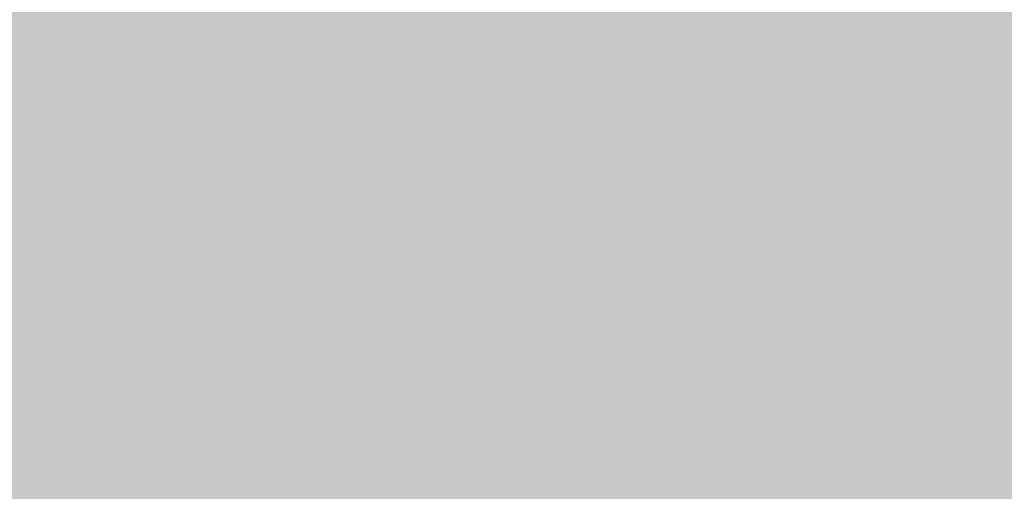
# Model space of a CAD drawing. Units: millimetres. Extents: x 0 to 2267, y 0 to 1823.
# Tile 224 of 256: x 1841.442 to 1842.748, y 1127.775 to 1128.399. Entities that reach past the tile are written whole.
import ezdxf

# ---------------------------------------------------------------- set-up
doc = ezdxf.new("R2010")
doc.units = ezdxf.units.MM
doc.header["$MEASUREMENT"] = 0
doc.layers.add('M-HATC', color=252, linetype='Continuous', lineweight=18)

msp = doc.modelspace()

# ---------------------------------------------------------------- hatches: boundary and pattern name
at = {"layer": 'M-HATC'}
h = msp.add_hatch(color=256, dxfattribs=at)
h.dxf.hatch_style = 1
h.paths.add_polyline_path([(2055.771, 1603.062), (1381.0868, 1603.062), (1381.0868, 1598.062), (2055.771, 1598.062)])
h.paths.add_polyline_path([(2055.771, 1598.062), (1381.0868, 1598.062), (1381.0868, 1593.062), (2055.771, 1593.062)])
h.paths.add_polyline_path([(2051.3074, 1536.7609), (1385.5504, 1536.7609), (1385.5504, 1526.7609), (1387.5504, 1526.7609), (1388.5366, 1525.0528), (1385.3319, 1521.2335), (1385.3319, 1521.2226), (2050.2542, 1522.7491), (2048.3212, 1525.0528), (2049.3074, 1526.7609), (2051.3074, 1526.7609)])
edge = h.paths.add_edge_path()
edge.add_arc((1847.5345, 1379.1492), 135, 222.603061, 222.890851, ccw=False)
edge.add_line((1748.1663, 1287.7656), (1683.0921, 1287.7656))
edge.add_arc((1583.7239, 1379.1492), 135, 317.109149, 317.396939, ccw=False)
edge.add_arc((1678.9686, 1290.6707), 5, 222.8909, 317.1091, ccw=False)
edge.add_arc((1774.2133, 1379.1492), 135, 222.603061, 222.890851, ccw=False)
edge.add_line((1674.8451, 1287.7656), (1609.7709, 1287.7656))
edge.add_arc((1510.4027, 1379.1492), 135, 317.109149, 317.396939, ccw=False)
edge.add_arc((1605.6474, 1290.6707), 5, 222.8909, 317.1091, ccw=False)
edge.add_arc((1700.8921, 1379.1492), 135, 222.603061, 222.890851, ccw=False)
edge.add_line((1601.5239, 1287.7656), (1536.4497, 1287.7656))
edge.add_arc((1437.0815, 1379.1492), 135, 317.109149, 317.396939, ccw=False)
edge.add_arc((1532.3262, 1290.6707), 5, 222.8909, 317.1091, ccw=False)
edge.add_arc((1627.5709, 1379.1492), 135, 222.603061, 222.890851, ccw=False)
edge.add_line((1528.2027, 1287.7656), (1505.9289, 1287.7656))
edge.add_spline(control_points=[(1505.9289, 1287.7656), (1504.2622, 1287.7656), (1504.2622, 1282.7656), (1505.9289, 1282.7656)], knot_values=[0, 0, 0, 0, 5, 5, 5, 5], degree=3, periodic=0)
edge.add_line((1505.9289, 1282.7656), (1930.9289, 1282.7656))
edge.add_spline(control_points=[(1930.9289, 1282.7656), (1932.5956, 1282.7656), (1932.5956, 1287.7656), (1930.9289, 1287.7656)], knot_values=[0, 0, 0, 0, 5, 5, 5, 5], degree=3, periodic=0)
edge.add_line((1930.9289, 1287.7656), (1903.0557, 1287.7656))
edge.add_arc((1803.6875, 1379.1492), 135, 317.109149, 317.396939, ccw=False)
edge.add_arc((1898.9322, 1290.6707), 5, 222.8909, 317.1091, ccw=False)
edge.add_arc((1994.1769, 1379.1492), 135, 222.603061, 222.890851, ccw=False)
edge.add_line((1894.8087, 1287.7656), (1829.7345, 1287.7656))
edge.add_arc((1730.3663, 1379.1492), 135, 317.109149, 317.396939, ccw=False)
edge.add_arc((1825.611, 1290.6707), 5, 222.8909, 317.1091, ccw=False)
edge.add_arc((1920.8557, 1379.1492), 135, 222.603061, 222.890851, ccw=False)
edge.add_line((1821.4875, 1287.7656), (1756.4133, 1287.7656))
edge.add_arc((1657.0451, 1379.1492), 135, 317.109149, 317.396939, ccw=False)
edge.add_arc((1752.2898, 1290.6707), 5, 222.8909, 317.1091, ccw=False)
edge = h.paths.add_edge_path()
edge.add_spline(control_points=[(1843.4289, 1227.2475), (1845.0956, 1227.2475), (1845.0956, 1232.2475), (1843.4289, 1232.2475)], knot_values=[0, 0, 0, 0, 5, 5, 5, 5], degree=3, periodic=0)
edge.add_line((1843.4289, 1232.2475), (1593.4289, 1232.2475))
edge.add_spline(control_points=[(1593.4289, 1232.2475), (1591.7622, 1232.2475), (1591.7622, 1227.2475), (1593.4289, 1227.2475)], knot_values=[0, 0, 0, 0, 5, 5, 5, 5], degree=3, periodic=0)
edge.add_line((1593.4289, 1227.2475), (1843.4289, 1227.2475))
h.paths.add_polyline_path([(1905.9289, 1127.4171), (1530.9289, 1127.4171, 0.414214), (1520.9289, 1117.4171), (1530.9289, 1117.4171), (1915.9289, 1117.4171, 0.414214)])
edge = h.paths.add_edge_path()
edge.add_arc((1397.0858, 1498.4078), 12.7299, 90.78215, 190.87871, ccw=False)
edge.add_line((1396.912, 1511.1365), (1428.0097, 1511.3488))
edge.add_line((1428.0097, 1511.3488), (1433.0097, 1511.3488))
edge.add_line((1433.0097, 1511.3488), (1434.439, 1511.3488))
edge.add_arc((1419.474, 1498.0804), 20, 41.561, 74.08211)
edge.add_line((1424.9592, 1517.3135), (1399.9351, 1517.2561))
edge.add_spline(control_points=[(1399.9307, 1517.2561), (1399.884, 1517.2131), (1399.8328, 1517.1689), (1399.7774, 1517.1236)], knot_values=[11.567499, 11.567499, 11.567499, 11.567499, 11.814249, 11.814249, 11.814249, 11.814249], degree=3, periodic=0)
edge.add_spline(control_points=[(1399.6328, 1517.0099), (1399.5831, 1516.9721), (1399.5307, 1516.9338), (1399.4759, 1516.8947)], knot_values=[11.167718, 11.167718, 11.167718, 11.167718, 11.365188, 11.365188, 11.365188, 11.365188], degree=3, periodic=0)
edge.add_spline(control_points=[(1399.3398, 1516.8001), (1399.1514, 1516.6719), (1398.9384, 1516.5377), (1398.704, 1516.3994)], knot_values=[10.376405, 10.376405, 10.376405, 10.376405, 11.00994, 11.00994, 11.00994, 11.00994], degree=3, periodic=0)
edge.add_spline(control_points=[(1398.6572, 1516.3719), (1398.5789, 1516.326), (1398.4983, 1516.2797), (1398.4155, 1516.2331)], knot_values=[10.125175, 10.125175, 10.125175, 10.125175, 10.334406, 10.334406, 10.334406, 10.334406], degree=3, periodic=0)
edge.add_spline(control_points=[(1398.2642, 1516.1487), (1398.196, 1516.1111), (1398.1263, 1516.0732), (1398.0555, 1516.0351)], knot_values=[9.832246, 9.832246, 9.832246, 9.832246, 9.999658, 9.999658, 9.999658, 9.999658], degree=3, periodic=0)
edge.add_spline(control_points=[(1397.9987, 1516.0048), (1397.7312, 1515.8621), (1397.446, 1515.7171), (1397.1466, 1515.5714)], knot_values=[9.161808, 9.161808, 9.161808, 9.161808, 9.787769, 9.787769, 9.787769, 9.787769], degree=3, periodic=0)
edge.add_spline(control_points=[(1397.1466, 1515.5714), (1396.8418, 1515.423), (1396.5222, 1515.274), (1396.1914, 1515.1262)], knot_values=[8.524455, 8.524455, 8.524455, 8.524455, 9.161808, 9.161808, 9.161808, 9.161808], degree=3, periodic=0)
edge.add_spline(control_points=[(1396.0777, 1515.0756), (1395.9854, 1515.0348), (1395.8922, 1514.994), (1395.7983, 1514.9534)], knot_values=[8.275193, 8.275193, 8.275193, 8.275193, 8.451726, 8.451726, 8.451726, 8.451726], degree=3, periodic=0)
edge.add_spline(control_points=[(1395.6018, 1514.8691), (1395.4997, 1514.8257), (1395.3968, 1514.7824), (1395.2932, 1514.7394)], knot_values=[7.962917, 7.962917, 7.962917, 7.962917, 8.152764, 8.152764, 8.152764, 8.152764], degree=3, periodic=0)
edge.add_spline(control_points=[(1395.2116, 1514.7057), (1394.8278, 1514.5475), (1394.4345, 1514.3929), (1394.0364, 1514.2442)], knot_values=[7.21254, 7.21254, 7.21254, 7.21254, 7.913148, 7.913148, 7.913148, 7.913148], degree=3, periodic=0)
edge.add_spline(control_points=[(1394.0364, 1514.2442), (1393.7076, 1514.1214), (1393.3754, 1514.0027), (1393.0427, 1513.8895)], knot_values=[6.633733, 6.633733, 6.633733, 6.633733, 7.21254, 7.21254, 7.21254, 7.21254], degree=3, periodic=0)
edge.add_spline(control_points=[(1392.8214, 1513.815), (1392.7198, 1513.7812), (1392.6181, 1513.7479), (1392.5166, 1513.7152)], knot_values=[6.328796, 6.328796, 6.328796, 6.328796, 6.505493, 6.505493, 6.505493, 6.505493], degree=3, periodic=0)
edge.add_spline(control_points=[(1392.5166, 1513.7152), (1392.3187, 1513.6515), (1392.1212, 1513.59), (1391.9244, 1513.531)], knot_values=[5.984605, 5.984605, 5.984605, 5.984605, 6.328796, 6.328796, 6.328796, 6.328796], degree=3, periodic=0)
edge.add_spline(control_points=[(1391.7915, 1513.4915), (1391.3122, 1513.3501), (1390.8384, 1513.2239), (1390.3784, 1513.1171)], knot_values=[5.066697, 5.066697, 5.066697, 5.066697, 5.907055, 5.907055, 5.907055, 5.907055], degree=3, periodic=0)
edge.add_spline(control_points=[(1390.3784, 1513.1171), (1390.1797, 1513.071), (1389.9836, 1513.0284), (1389.7907, 1512.9899)], knot_values=[4.70367, 4.70367, 4.70367, 4.70367, 5.066695, 5.066695, 5.066695, 5.066695], degree=3, periodic=0)
edge.add_spline(control_points=[(1389.422, 1512.9204), (1389.2459, 1512.8892), (1389.0729, 1512.8617), (1388.9036, 1512.8381)], knot_values=[4.130571, 4.130571, 4.130571, 4.130571, 4.469816, 4.469816, 4.469816, 4.469816], degree=3, periodic=0)
edge.add_spline(control_points=[(1388.9036, 1512.8381), (1388.591, 1512.7946), (1388.2911, 1512.7644), (1388.0071, 1512.7494)], knot_values=[3.504031, 3.504031, 3.504031, 3.504031, 4.130571, 4.130571, 4.130571, 4.130571], degree=3, periodic=0)
edge.add_spline(control_points=[(1387.9356, 1512.7459), (1387.8538, 1512.7423), (1387.7733, 1512.74), (1387.6944, 1512.739)], knot_values=[3.268866, 3.268866, 3.268866, 3.268866, 3.451164, 3.451164, 3.451164, 3.451164], degree=3, periodic=0)
edge.add_spline(control_points=[(1387.3351, 1512.7443), (1387.2076, 1512.7499), (1387.0847, 1512.7597), (1386.967, 1512.7739)], knot_values=[2.670686, 2.670686, 2.670686, 2.670686, 2.984, 2.984, 2.984, 2.984], degree=3, periodic=0)
edge.add_spline(control_points=[(1386.8327, 1512.7922), (1386.8209, 1512.7941), (1386.8092, 1512.7959), (1386.7975, 1512.7979)], knot_values=[2.516981, 2.516981, 2.516981, 2.516981, 2.549528, 2.549528, 2.549528, 2.549528], degree=3, periodic=0)
edge.add_spline(control_points=[(1386.4526, 1512.8735), (1386.4257, 1512.881), (1386.3993, 1512.889), (1386.3733, 1512.8972)], knot_values=[2.095869, 2.095869, 2.095869, 2.095869, 2.17941, 2.17941, 2.17941, 2.17941], degree=3, periodic=0)
edge.add_spline(control_points=[(1386.0691, 1513.0189), (1386.0634, 1513.0217), (1386.0577, 1513.0246), (1386.052, 1513.0275)], knot_values=[1.72453, 1.72453, 1.72453, 1.72453, 1.745933, 1.745933, 1.745933, 1.745933], degree=3, periodic=0)
edge.add_arc((1399.474, 1498.0804), 20, 131.82432, 180)
edge.add_arc((1630.3336, 1505.5484), 250.9708, 181.705176, 236.427975)
edge.add_arc((1605.3399, 1483.3044), 218.7822, 238.660829, 243.34961)
edge.add_arc((1647.0911, 1510.3592), 262.8986, 183.129836, 237.853442, ccw=False)
h.paths.add_polyline_path([(1406.5369, 1391.9644, 0.149382), (1491.5506, 1296.4418, -0.129517)], flags=17)
edge = h.paths.add_edge_path()
edge.add_arc((2037.3838, 1498.0804), 20, 0, 48.26587)
edge.add_spline(control_points=[(2050.6973, 1513.0052), (2050.6512, 1512.9847), (2050.6034, 1512.9655), (2050.5539, 1512.9477)], knot_values=[1.835652, 1.835652, 1.835652, 1.835652, 2.000781, 2.000781, 2.000781, 2.000781], degree=3, periodic=0)
edge.add_spline(control_points=[(2050.4616, 1512.9166), (2050.479, 1512.9221), (2050.4963, 1512.9277), (2050.5133, 1512.9335)], knot_values=[2.045477, 2.045477, 2.045477, 2.045477, 2.101389, 2.101389, 2.101389, 2.101389], degree=3, periodic=0)
edge.add_spline(control_points=[(2050.129, 1512.8342), (2050.1984, 1512.8473), (2050.2657, 1512.8623), (2050.3308, 1512.8792)], knot_values=[2.237629, 2.237629, 2.237629, 2.237629, 2.435841, 2.435841, 2.435841, 2.435841], degree=3, periodic=0)
edge.add_spline(control_points=[(2050.0946, 1512.8278), (2050.1061, 1512.8299), (2050.1176, 1512.832), (2050.129, 1512.8342)], knot_values=[2.435841, 2.435841, 2.435841, 2.435841, 2.468321, 2.468321, 2.468321, 2.468321], degree=3, periodic=0)
edge.add_spline(control_points=[(2049.7843, 1512.7851), (2049.8552, 1512.7922), (2049.9243, 1512.8008), (2049.9917, 1512.8109)], knot_values=[2.563852, 2.563852, 2.563852, 2.563852, 2.748541, 2.748541, 2.748541, 2.748541], degree=3, periodic=0)
edge.add_spline(control_points=[(2049.4052, 1512.7617), (2049.5364, 1512.7653), (2049.6629, 1512.773), (2049.7843, 1512.7851)], knot_values=[2.748541, 2.748541, 2.748541, 2.748541, 3.064882, 3.064882, 3.064882, 3.064882], degree=3, periodic=0)
edge.add_spline(control_points=[(2049.1698, 1512.7597), (2049.2336, 1512.7591), (2049.2965, 1512.7594), (2049.3584, 1512.7606)], knot_values=[3.102309, 3.102309, 3.102309, 3.102309, 3.2503, 3.2503, 3.2503, 3.2503], degree=3, periodic=0)
edge.add_spline(control_points=[(2048.8573, 1512.7691), (2048.9638, 1512.7638), (2049.068, 1512.7606), (2049.1698, 1512.7597)], knot_values=[3.2503, 3.2503, 3.2503, 3.2503, 3.486069, 3.486069, 3.486069, 3.486069], degree=3, periodic=0)
edge.add_spline(control_points=[(2048.6924, 1512.7789), (2048.3729, 1512.8009), (2048.0345, 1512.8411), (2047.6817, 1512.897)], knot_values=[3.606429, 3.606429, 3.606429, 3.606429, 4.2989, 4.2989, 4.2989, 4.2989], degree=3, periodic=0)
edge.add_spline(control_points=[(2047.6817, 1512.897), (2047.5458, 1512.9185), (2047.4077, 1512.9424), (2047.2678, 1512.9685)], knot_values=[4.2989, 4.2989, 4.2989, 4.2989, 4.565769, 4.565769, 4.565769, 4.565769], degree=3, periodic=0)
edge.add_spline(control_points=[(2047.2678, 1512.9685), (2047.1449, 1512.9914), (2047.0207, 1513.016), (2046.8951, 1513.0422)], knot_values=[4.565769, 4.565769, 4.565769, 4.565769, 4.799971, 4.799971, 4.799971, 4.799971], degree=3, periodic=0)
edge.add_spline(control_points=[(2046.8951, 1513.0422), (2046.5286, 1513.1188), (2046.1513, 1513.209), (2045.7676, 1513.3107)], knot_values=[4.799971, 4.799971, 4.799971, 4.799971, 5.483718, 5.483718, 5.483718, 5.483718], degree=3, periodic=0)
edge.add_spline(control_points=[(2045.7676, 1513.3107), (2045.3724, 1513.4154), (2044.9704, 1513.5322), (2044.5662, 1513.6588)], knot_values=[5.483718, 5.483718, 5.483718, 5.483718, 6.187866, 6.187866, 6.187866, 6.187866], degree=3, periodic=0)
edge.add_spline(control_points=[(2044.5662, 1513.6588), (2044.4149, 1513.7061), (2044.2633, 1513.7549), (2044.1116, 1513.8048)], knot_values=[6.187866, 6.187866, 6.187866, 6.187866, 6.451551, 6.451551, 6.451551, 6.451551], degree=3, periodic=0)
edge.add_spline(control_points=[(2044.1116, 1513.8048), (2043.9967, 1513.8427), (2043.8817, 1513.8813), (2043.7668, 1513.9205)], knot_values=[6.451551, 6.451551, 6.451551, 6.451551, 6.651434, 6.651434, 6.651434, 6.651434], degree=3, periodic=0)
edge.add_spline(control_points=[(2043.7668, 1513.9205), (2043.3716, 1514.0554), (2042.9774, 1514.1979), (2042.5886, 1514.3458)], knot_values=[6.651434, 6.651434, 6.651434, 6.651434, 7.338879, 7.338879, 7.338879, 7.338879], degree=3, periodic=0)
edge.add_spline(control_points=[(2042.5886, 1514.3458), (2042.1643, 1514.5071), (2041.7465, 1514.6749), (2041.3409, 1514.846)], knot_values=[7.338879, 7.338879, 7.338879, 7.338879, 8.089209, 8.089209, 8.089209, 8.089209], degree=3, periodic=0)
edge.add_spline(control_points=[(2041.3409, 1514.846), (2041.1028, 1514.9465), (2040.869, 1515.0481), (2040.6405, 1515.1502)], knot_values=[8.089209, 8.089209, 8.089209, 8.089209, 8.529587, 8.529587, 8.529587, 8.529587], degree=3, periodic=0)
edge.add_spline(control_points=[(2040.51, 1515.2089), (2040.0824, 1515.4022), (2039.6747, 1515.5971), (2039.295, 1515.7894)], knot_values=[8.613818, 8.613818, 8.613818, 8.613818, 9.44571, 9.44571, 9.44571, 9.44571], degree=3, periodic=0)
edge.add_spline(control_points=[(2039.295, 1515.7894), (2039.0618, 1515.9075), (2038.8391, 1516.0246), (2038.6288, 1516.1398)], knot_values=[9.44571, 9.44571, 9.44571, 9.44571, 9.956404, 9.956404, 9.956404, 9.956404], degree=3, periodic=0)
edge.add_spline(control_points=[(2038.6288, 1516.1398), (2038.5187, 1516.2001), (2038.4121, 1516.2598), (2038.309, 1516.3189)], knot_values=[9.956404, 9.956404, 9.956404, 9.956404, 10.223542, 10.223542, 10.223542, 10.223542], degree=3, periodic=0)
edge.add_spline(control_points=[(2038.309, 1516.3189), (2038.2138, 1516.3735), (2038.1216, 1516.4276), (2038.0328, 1516.481)], knot_values=[10.223542, 10.223542, 10.223542, 10.223542, 10.47051, 10.47051, 10.47051, 10.47051], degree=3, periodic=0)
edge.add_spline(control_points=[(2038.0328, 1516.481), (2037.7855, 1516.6296), (2037.5639, 1516.773), (2037.3722, 1516.909)], knot_values=[10.47051, 10.47051, 10.47051, 10.47051, 11.15767, 11.15767, 11.15767, 11.15767], degree=3, periodic=0)
edge.add_spline(control_points=[(2037.3722, 1516.909), (2037.2789, 1516.9752), (2037.1927, 1517.0396), (2037.1142, 1517.102)], knot_values=[11.15767, 11.15767, 11.15767, 11.15767, 11.49227, 11.49227, 11.49227, 11.49227], degree=3, periodic=0)
edge.add_spline(control_points=[(2036.8564, 1517.3259), (2036.9148, 1517.2692), (2036.9814, 1517.2103), (2037.0557, 1517.1492)], knot_values=[11.577341, 11.577341, 11.577341, 11.577341, 11.91035, 11.91035, 11.91035, 11.91035], degree=3, periodic=0)
edge.add_spline(control_points=[(2036.8074, 1517.3748), (2036.823, 1517.3587), (2036.8393, 1517.3424), (2036.8564, 1517.3259)], knot_values=[11.91035, 11.91035, 11.91035, 11.91035, 12.007402, 12.007402, 12.007402, 12.007402], degree=3, periodic=0)
edge.add_spline(control_points=[(2036.7017, 1517.494), (2036.7104, 1517.483), (2036.7196, 1517.4719), (2036.7291, 1517.4606)], knot_values=[12.184155, 12.184155, 12.184155, 12.184155, 12.255409, 12.255409, 12.255409, 12.255409], degree=3, periodic=0)
edge.add_spline(control_points=[(2036.6159, 1517.6205), (2036.62, 1517.613), (2036.6243, 1517.6055), (2036.6289, 1517.5979)], knot_values=[12.487913, 12.487913, 12.487913, 12.487913, 12.541035, 12.541035, 12.541035, 12.541035], degree=3, periodic=0)
edge.add_spline(control_points=[(2036.5635, 1517.786), (2036.5637, 1517.7794), (2036.5642, 1517.7726), (2036.565, 1517.7658)], knot_values=[12.911761, 12.911761, 12.911761, 12.911761, 12.968286, 12.968286, 12.968286, 12.968286], degree=3, periodic=0)
edge.add_spline(control_points=[(2036.6166, 1517.9304), (2036.6125, 1517.9259), (2036.6086, 1517.9212), (2036.6049, 1517.9165)], knot_values=[13.382527, 13.382527, 13.382527, 13.382527, 13.433791, 13.433791, 13.433791, 13.433791], degree=3, periodic=0)
edge.add_spline(control_points=[(2036.749, 1518.017), (2036.7361, 1518.0116), (2036.7239, 1518.006), (2036.7124, 1518.0002)], knot_values=[13.726299, 13.726299, 13.726299, 13.726299, 13.809928, 13.809928, 13.809928, 13.809928], degree=3, periodic=0)
edge.add_spline(control_points=[(2036.8604, 1518.0528), (2036.8386, 1518.0474), (2036.8181, 1518.0416), (2036.7988, 1518.0353)], knot_values=[13.910887, 13.910887, 13.910887, 13.910887, 14.02153, 14.02153, 14.02153, 14.02153], degree=3, periodic=0)
edge.add_line((2036.9639, 1518.0804), (2032.3838, 1518.0804))
edge.add_line((2032.3838, 1518.0804), (2027.3838, 1518.0804))
edge.add_line((2027.3838, 1518.0804), (2022.3838, 1518.0804))
edge.add_line((2022.3838, 1518.0804), (2017.3838, 1518.0804))
edge.add_arc((2017.3838, 1498.0804), 20, 90, 138.439)
edge.add_line((2002.4188, 1511.3488), (2003.8481, 1511.3488))
edge.add_line((2003.8481, 1511.3488), (2008.8481, 1511.3488))
edge.add_line((2008.8481, 1511.3488), (2039.772, 1511.1377))
edge.add_arc((2039.772, 1498.4078), 12.7299, -10.87871, 90, ccw=False)
edge.add_arc((1789.7668, 1510.3592), 262.8986, 302.146558, 356.870164, ccw=False)
edge.add_arc((1831.5179, 1483.3044), 218.7822, 296.65039, 301.339171)
edge.add_arc((1806.5242, 1505.5484), 250.9708, 303.572025, 358.294824)
h.paths.add_polyline_path([(2030.321, 1391.9644, -0.129517), (1945.3072, 1296.4418, 0.149382)], flags=17)
edge = h.paths.add_edge_path()
edge.add_spline(control_points=[(2037.2464, 1518.0821), (2037.2898, 1518.081), (2037.3355, 1518.0804), (2037.3838, 1518.0804)], knot_values=[0.000012, 0.000012, 0.000012, 0.000012, 0.144754, 0.144754, 0.144754, 0.144754], degree=3, periodic=0)
edge.add_line((2037.3357, 1518.0804), (2037.0096, 1518.0804))
edge.add_spline(control_points=[(2037.0096, 1518.0804), (2036.9822, 1518.0768), (2036.956, 1518.0727), (2036.9312, 1518.0681)], knot_values=[14.13465, 14.13465, 14.13465, 14.13465, 14.247197, 14.247197, 14.247197, 14.247197], degree=3, periodic=0)
edge.add_spline(control_points=[(2036.9312, 1518.0681), (2036.9276, 1518.0674), (2036.9241, 1518.0667), (2036.9205, 1518.0661)], knot_values=[14.118315, 14.118315, 14.118315, 14.118315, 14.13465, 14.13465, 14.13465, 14.13465], degree=3, periodic=0)
edge.add_spline(control_points=[(2036.9205, 1518.0661), (2036.9118, 1518.0644), (2036.9032, 1518.0626), (2036.8948, 1518.0608)], knot_values=[14.078086, 14.078086, 14.078086, 14.078086, 14.118315, 14.118315, 14.118315, 14.118315], degree=3, periodic=0)
edge.add_spline(control_points=[(2036.8948, 1518.0608), (2036.883, 1518.0583), (2036.8716, 1518.0556), (2036.8604, 1518.0528)], knot_values=[14.02153, 14.02153, 14.02153, 14.02153, 14.078086, 14.078086, 14.078086, 14.078086], degree=3, periodic=0)
edge.add_spline(control_points=[(2036.8604, 1518.0528), (2036.8386, 1518.0474), (2036.8181, 1518.0416), (2036.7988, 1518.0353)], knot_values=[13.910887, 13.910887, 13.910887, 13.910887, 14.02153, 14.02153, 14.02153, 14.02153], degree=3, periodic=0)
edge.add_spline(control_points=[(2036.7988, 1518.0353), (2036.7981, 1518.035), (2036.7974, 1518.0348), (2036.7967, 1518.0346)], knot_values=[13.906906, 13.906906, 13.906906, 13.906906, 13.910887, 13.910887, 13.910887, 13.910887], degree=3, periodic=0)
edge.add_spline(control_points=[(2036.7967, 1518.0346), (2036.7882, 1518.0318), (2036.7799, 1518.0289), (2036.7719, 1518.0259)], knot_values=[13.857826, 13.857826, 13.857826, 13.857826, 13.906906, 13.906906, 13.906906, 13.906906], degree=3, periodic=0)
edge.add_spline(control_points=[(2036.7719, 1518.0259), (2036.764, 1518.023), (2036.7564, 1518.02), (2036.749, 1518.017)], knot_values=[13.809928, 13.809928, 13.809928, 13.809928, 13.857826, 13.857826, 13.857826, 13.857826], degree=3, periodic=0)
edge.add_spline(control_points=[(2036.749, 1518.017), (2036.7361, 1518.0116), (2036.7239, 1518.006), (2036.7124, 1518.0002)], knot_values=[13.726299, 13.726299, 13.726299, 13.726299, 13.809928, 13.809928, 13.809928, 13.809928], degree=3, periodic=0)
edge.add_spline(control_points=[(2036.7124, 1518.0002), (2036.7121, 1518), (2036.7118, 1517.9999), (2036.7115, 1517.9997)], knot_values=[13.723993, 13.723993, 13.723993, 13.723993, 13.726299, 13.726299, 13.726299, 13.726299], degree=3, periodic=0)
edge.add_spline(control_points=[(2036.7115, 1517.9997), (2036.7063, 1517.9971), (2036.7013, 1517.9944), (2036.6965, 1517.9917)], knot_values=[13.686536, 13.686536, 13.686536, 13.686536, 13.723993, 13.723993, 13.723993, 13.723993], degree=3, periodic=0)
edge.add_spline(control_points=[(2036.6965, 1517.9917), (2036.6919, 1517.9891), (2036.6874, 1517.9865), (2036.6831, 1517.9839)], knot_values=[13.651251, 13.651251, 13.651251, 13.651251, 13.686536, 13.686536, 13.686536, 13.686536], degree=3, periodic=0)
edge.add_spline(control_points=[(2036.6831, 1517.9839), (2036.6764, 1517.9798), (2036.67, 1517.9757), (2036.6639, 1517.9714)], knot_values=[13.596804, 13.596804, 13.596804, 13.596804, 13.651251, 13.651251, 13.651251, 13.651251], degree=3, periodic=0)
edge.add_spline(control_points=[(2036.6639, 1517.9714), (2036.6636, 1517.9712), (2036.6633, 1517.9709), (2036.6629, 1517.9707)], knot_values=[13.593956, 13.593956, 13.593956, 13.593956, 13.596804, 13.596804, 13.596804, 13.596804], degree=3, periodic=0)
edge.add_spline(control_points=[(2036.6629, 1517.9707), (2036.6603, 1517.9689), (2036.6577, 1517.967), (2036.6552, 1517.9651)], knot_values=[13.570322, 13.570322, 13.570322, 13.570322, 13.593956, 13.593956, 13.593956, 13.593956], degree=3, periodic=0)
edge.add_spline(control_points=[(2036.6552, 1517.9651), (2036.6525, 1517.9631), (2036.6499, 1517.9611), (2036.6474, 1517.9591)], knot_values=[13.545477, 13.545477, 13.545477, 13.545477, 13.570322, 13.570322, 13.570322, 13.570322], degree=3, periodic=0)
edge.add_spline(control_points=[(2036.6474, 1517.9591), (2036.6472, 1517.9589), (2036.6471, 1517.9588), (2036.6469, 1517.9587)], knot_values=[13.543931, 13.543931, 13.543931, 13.543931, 13.545477, 13.545477, 13.545477, 13.545477], degree=3, periodic=0)
edge.add_spline(control_points=[(2036.6469, 1517.9587), (2036.6412, 1517.9541), (2036.6358, 1517.9494), (2036.6307, 1517.9447)], knot_values=[13.488237, 13.488237, 13.488237, 13.488237, 13.543931, 13.543931, 13.543931, 13.543931], degree=3, periodic=0)
edge.add_spline(control_points=[(2036.6307, 1517.9447), (2036.6282, 1517.9423), (2036.6257, 1517.9399), (2036.6233, 1517.9374)], knot_values=[13.460307, 13.460307, 13.460307, 13.460307, 13.488237, 13.488237, 13.488237, 13.488237], degree=3, periodic=0)
edge.add_spline(control_points=[(2036.6233, 1517.9374), (2036.6215, 1517.9356), (2036.6198, 1517.9338), (2036.6181, 1517.932)], knot_values=[13.439712, 13.439712, 13.439712, 13.439712, 13.460307, 13.460307, 13.460307, 13.460307], degree=3, periodic=0)
edge.add_spline(control_points=[(2036.6181, 1517.932), (2036.6176, 1517.9315), (2036.6171, 1517.9309), (2036.6166, 1517.9304)], knot_values=[13.433791, 13.433791, 13.433791, 13.433791, 13.439712, 13.439712, 13.439712, 13.439712], degree=3, periodic=0)
edge.add_spline(control_points=[(2036.6166, 1517.9304), (2036.6125, 1517.9259), (2036.6086, 1517.9212), (2036.6049, 1517.9165)], knot_values=[13.382527, 13.382527, 13.382527, 13.382527, 13.433791, 13.433791, 13.433791, 13.433791], degree=3, periodic=0)
edge.add_spline(control_points=[(2036.6049, 1517.9165), (2036.6026, 1517.9135), (2036.6004, 1517.9104), (2036.5982, 1517.9074)], knot_values=[13.350017, 13.350017, 13.350017, 13.350017, 13.382527, 13.382527, 13.382527, 13.382527], degree=3, periodic=0)
edge.add_spline(control_points=[(2036.5982, 1517.9074), (2036.5972, 1517.9059), (2036.5962, 1517.9043), (2036.5952, 1517.9028)], knot_values=[13.333922, 13.333922, 13.333922, 13.333922, 13.350017, 13.350017, 13.350017, 13.350017], degree=3, periodic=0)
edge.add_spline(control_points=[(2036.5952, 1517.9028), (2036.5945, 1517.9018), (2036.5939, 1517.9009), (2036.5933, 1517.8999)], knot_values=[13.323828, 13.323828, 13.323828, 13.323828, 13.333922, 13.333922, 13.333922, 13.333922], degree=3, periodic=0)
edge.add_spline(control_points=[(2036.5933, 1517.8999), (2036.5905, 1517.8955), (2036.5879, 1517.8909), (2036.5855, 1517.8864)], knot_values=[13.277545, 13.277545, 13.277545, 13.277545, 13.323828, 13.323828, 13.323828, 13.323828], degree=3, periodic=0)
edge.add_spline(control_points=[(2036.5855, 1517.8864), (2036.5836, 1517.8827), (2036.5817, 1517.8789), (2036.5801, 1517.8751)], knot_values=[13.240119, 13.240119, 13.240119, 13.240119, 13.277545, 13.277545, 13.277545, 13.277545], degree=3, periodic=0)
edge.add_spline(control_points=[(2036.5801, 1517.8751), (2036.5795, 1517.8739), (2036.579, 1517.8727), (2036.5785, 1517.8715)], knot_values=[13.228211, 13.228211, 13.228211, 13.228211, 13.240119, 13.240119, 13.240119, 13.240119], degree=3, periodic=0)
edge.add_spline(control_points=[(2036.5785, 1517.8715), (2036.578, 1517.8702), (2036.5774, 1517.869), (2036.5769, 1517.8677)], knot_values=[13.215717, 13.215717, 13.215717, 13.215717, 13.228211, 13.228211, 13.228211, 13.228211], degree=3, periodic=0)
edge.add_spline(control_points=[(2036.5769, 1517.8677), (2036.5755, 1517.864), (2036.5741, 1517.8603), (2036.5729, 1517.8565)], knot_values=[13.179847, 13.179847, 13.179847, 13.179847, 13.215717, 13.215717, 13.215717, 13.215717], degree=3, periodic=0)
edge.add_spline(control_points=[(2036.5729, 1517.8565), (2036.5713, 1517.8515), (2036.5699, 1517.8464), (2036.5687, 1517.8413)], knot_values=[13.132017, 13.132017, 13.132017, 13.132017, 13.179847, 13.179847, 13.179847, 13.179847], degree=3, periodic=0)
edge.add_spline(control_points=[(2036.5687, 1517.8413), (2036.5684, 1517.8402), (2036.5682, 1517.8392), (2036.568, 1517.8382)], knot_values=[13.122482, 13.122482, 13.122482, 13.122482, 13.132017, 13.132017, 13.132017, 13.132017], degree=3, periodic=0)
edge.add_spline(control_points=[(2036.568, 1517.8382), (2036.5676, 1517.8363), (2036.5672, 1517.8345), (2036.5669, 1517.8327)], knot_values=[13.105592, 13.105592, 13.105592, 13.105592, 13.122482, 13.122482, 13.122482, 13.122482], degree=3, periodic=0)
edge.add_spline(control_points=[(2036.5669, 1517.8327), (2036.5662, 1517.8292), (2036.5657, 1517.8257), (2036.5652, 1517.8222)], knot_values=[13.074063, 13.074063, 13.074063, 13.074063, 13.105592, 13.105592, 13.105592, 13.105592], degree=3, periodic=0)
edge.add_spline(control_points=[(2036.5652, 1517.8222), (2036.5652, 1517.8222), (2036.5652, 1517.8222), (2036.5652, 1517.8222)], knot_values=[13.074043, 13.074043, 13.074043, 13.074043, 13.074063, 13.074063, 13.074063, 13.074063], degree=3, periodic=0)
edge.add_spline(control_points=[(2036.5652, 1517.8222), (2036.5644, 1517.8164), (2036.5639, 1517.8106), (2036.5636, 1517.8046)], knot_values=[13.021884, 13.021884, 13.021884, 13.021884, 13.074043, 13.074043, 13.074043, 13.074043], degree=3, periodic=0)
edge.add_spline(control_points=[(2036.5636, 1517.8046), (2036.5636, 1517.804), (2036.5636, 1517.8034), (2036.5635, 1517.8028)], knot_values=[13.01674, 13.01674, 13.01674, 13.01674, 13.021884, 13.021884, 13.021884, 13.021884], degree=3, periodic=0)
edge.add_spline(control_points=[(2036.5635, 1517.8028), (2036.5634, 1517.8005), (2036.5634, 1517.7982), (2036.5634, 1517.7958)], knot_values=[12.996438, 12.996438, 12.996438, 12.996438, 13.01674, 13.01674, 13.01674, 13.01674], degree=3, periodic=0)
edge.add_spline(control_points=[(2036.5634, 1517.7958), (2036.5633, 1517.7926), (2036.5634, 1517.7893), (2036.5635, 1517.786)], knot_values=[12.968286, 12.968286, 12.968286, 12.968286, 12.996438, 12.996438, 12.996438, 12.996438], degree=3, periodic=0)
edge.add_spline(control_points=[(2036.5635, 1517.786), (2036.5637, 1517.7794), (2036.5642, 1517.7726), (2036.565, 1517.7658)], knot_values=[12.911761, 12.911761, 12.911761, 12.911761, 12.968286, 12.968286, 12.968286, 12.968286], degree=3, periodic=0)
edge.add_spline(control_points=[(2036.565, 1517.7658), (2036.565, 1517.7657), (2036.565, 1517.7656), (2036.565, 1517.7656)], knot_values=[12.911017, 12.911017, 12.911017, 12.911017, 12.911761, 12.911761, 12.911761, 12.911761], degree=3, periodic=0)
edge.add_spline(control_points=[(2036.565, 1517.7656), (2036.5654, 1517.7625), (2036.5658, 1517.7593), (2036.5663, 1517.7562)], knot_values=[12.88528, 12.88528, 12.88528, 12.88528, 12.911017, 12.911017, 12.911017, 12.911017], degree=3, periodic=0)
edge.add_spline(control_points=[(2036.5663, 1517.7562), (2036.5667, 1517.7534), (2036.5672, 1517.7506), (2036.5677, 1517.7478)], knot_values=[12.862519, 12.862519, 12.862519, 12.862519, 12.88528, 12.88528, 12.88528, 12.88528], degree=3, periodic=0)
edge.add_spline(control_points=[(2036.5677, 1517.7478), (2036.5678, 1517.7474), (2036.5679, 1517.7469), (2036.568, 1517.7465)], knot_values=[12.858885, 12.858885, 12.858885, 12.858885, 12.862519, 12.862519, 12.862519, 12.862519], degree=3, periodic=0)
edge.add_spline(control_points=[(2036.568, 1517.7465), (2036.5692, 1517.7399), (2036.5707, 1517.7332), (2036.5724, 1517.7264)], knot_values=[12.8053, 12.8053, 12.8053, 12.8053, 12.858885, 12.858885, 12.858885, 12.858885], degree=3, periodic=0)
edge.add_spline(control_points=[(2036.5724, 1517.7264), (2036.5734, 1517.7226), (2036.5745, 1517.7187), (2036.5756, 1517.7149)], knot_values=[12.775176, 12.775176, 12.775176, 12.775176, 12.8053, 12.8053, 12.8053, 12.8053], degree=3, periodic=0)
edge.add_spline(control_points=[(2036.5756, 1517.7149), (2036.5763, 1517.7125), (2036.577, 1517.7102), (2036.5778, 1517.7078)], knot_values=[12.756759, 12.756759, 12.756759, 12.756759, 12.775176, 12.775176, 12.775176, 12.775176], degree=3, periodic=0)
edge.add_spline(control_points=[(2036.5778, 1517.7078), (2036.5781, 1517.7067), (2036.5784, 1517.7057), (2036.5787, 1517.7047)], knot_values=[12.748742, 12.748742, 12.748742, 12.748742, 12.756759, 12.756759, 12.756759, 12.756759], degree=3, periodic=0)
edge.add_spline(control_points=[(2036.5787, 1517.7047), (2036.5808, 1517.6983), (2036.5831, 1517.6919), (2036.5856, 1517.6854)], knot_values=[12.69959, 12.69959, 12.69959, 12.69959, 12.748742, 12.748742, 12.748742, 12.748742], degree=3, periodic=0)
edge.add_spline(control_points=[(2036.5856, 1517.6854), (2036.5876, 1517.68), (2036.5898, 1517.6746), (2036.5921, 1517.6692)], knot_values=[12.659038, 12.659038, 12.659038, 12.659038, 12.69959, 12.69959, 12.69959, 12.69959], degree=3, periodic=0)
edge.add_spline(control_points=[(2036.5921, 1517.6692), (2036.594, 1517.6648), (2036.5959, 1517.6605), (2036.5979, 1517.6561)], knot_values=[12.626806, 12.626806, 12.626806, 12.626806, 12.659038, 12.659038, 12.659038, 12.659038], degree=3, periodic=0)
edge.add_spline(control_points=[(2036.5979, 1517.6561), (2036.5984, 1517.6551), (2036.5989, 1517.6541), (2036.5993, 1517.6531)], knot_values=[12.619394, 12.619394, 12.619394, 12.619394, 12.626806, 12.626806, 12.626806, 12.626806], degree=3, periodic=0)
edge.add_spline(control_points=[(2036.5993, 1517.6531), (2036.6043, 1517.6424), (2036.6099, 1517.6315), (2036.6159, 1517.6205)], knot_values=[12.541039, 12.541039, 12.541039, 12.541039, 12.619394, 12.619394, 12.619394, 12.619394], degree=3, periodic=0)
edge.add_spline(control_points=[(2036.6159, 1517.6205), (2036.6159, 1517.6205), (2036.6159, 1517.6205), (2036.6159, 1517.6205)], knot_values=[12.541035, 12.541035, 12.541035, 12.541035, 12.541039, 12.541039, 12.541039, 12.541039], degree=3, periodic=0)
edge.add_spline(control_points=[(2036.6159, 1517.6205), (2036.62, 1517.613), (2036.6243, 1517.6055), (2036.6289, 1517.5979)], knot_values=[12.487913, 12.487913, 12.487913, 12.487913, 12.541035, 12.541035, 12.541035, 12.541035], degree=3, periodic=0)
edge.add_spline(control_points=[(2036.6289, 1517.5979), (2036.6326, 1517.5916), (2036.6365, 1517.5853), (2036.6406, 1517.5789)], knot_values=[12.443982, 12.443982, 12.443982, 12.443982, 12.487913, 12.487913, 12.487913, 12.487913], degree=3, periodic=0)
edge.add_spline(control_points=[(2036.6406, 1517.5789), (2036.6414, 1517.5776), (2036.6423, 1517.5763), (2036.6431, 1517.5749)], knot_values=[12.434996, 12.434996, 12.434996, 12.434996, 12.443982, 12.443982, 12.443982, 12.443982], degree=3, periodic=0)
edge.add_spline(control_points=[(2036.6431, 1517.5749), (2036.6531, 1517.5596), (2036.6639, 1517.5439), (2036.6756, 1517.528)], knot_values=[12.329647, 12.329647, 12.329647, 12.329647, 12.434996, 12.434996, 12.434996, 12.434996], degree=3, periodic=0)
edge.add_spline(control_points=[(2036.6756, 1517.528), (2036.6839, 1517.5168), (2036.6925, 1517.5055), (2036.7017, 1517.494)], knot_values=[12.255409, 12.255409, 12.255409, 12.255409, 12.329647, 12.329647, 12.329647, 12.329647], degree=3, periodic=0)
edge.add_spline(control_points=[(2036.7017, 1517.494), (2036.7104, 1517.483), (2036.7196, 1517.4719), (2036.7291, 1517.4606)], knot_values=[12.184155, 12.184155, 12.184155, 12.184155, 12.255409, 12.255409, 12.255409, 12.255409], degree=3, periodic=0)
edge.add_spline(control_points=[(2036.7291, 1517.4606), (2036.7436, 1517.4435), (2036.759, 1517.4262), (2036.7753, 1517.4085)], knot_values=[12.075961, 12.075961, 12.075961, 12.075961, 12.184155, 12.184155, 12.184155, 12.184155], degree=3, periodic=0)
edge.add_spline(control_points=[(2036.7753, 1517.4085), (2036.7763, 1517.4075), (2036.7773, 1517.4064), (2036.7783, 1517.4054)], knot_values=[12.069502, 12.069502, 12.069502, 12.069502, 12.075961, 12.075961, 12.075961, 12.075961], degree=3, periodic=0)
edge.add_spline(control_points=[(2036.7783, 1517.4054), (2036.7877, 1517.3953), (2036.7974, 1517.385), (2036.8074, 1517.3748)], knot_values=[12.007402, 12.007402, 12.007402, 12.007402, 12.069502, 12.069502, 12.069502, 12.069502], degree=3, periodic=0)
edge.add_spline(control_points=[(2036.8074, 1517.3748), (2036.823, 1517.3587), (2036.8393, 1517.3424), (2036.8564, 1517.3259)], knot_values=[11.91035, 11.91035, 11.91035, 11.91035, 12.007402, 12.007402, 12.007402, 12.007402], degree=3, periodic=0)
edge.add_spline(control_points=[(2036.8564, 1517.3259), (2036.9148, 1517.2692), (2036.9814, 1517.2103), (2037.0557, 1517.1492)], knot_values=[11.577341, 11.577341, 11.577341, 11.577341, 11.91035, 11.91035, 11.91035, 11.91035], degree=3, periodic=0)
edge.add_spline(control_points=[(2037.0557, 1517.1492), (2037.0747, 1517.1336), (2037.0942, 1517.1179), (2037.1142, 1517.102)], knot_values=[11.49227, 11.49227, 11.49227, 11.49227, 11.577341, 11.577341, 11.577341, 11.577341], degree=3, periodic=0)
edge.add_spline(control_points=[(2037.1142, 1517.102), (2037.1927, 1517.0396), (2037.2789, 1516.9752), (2037.3722, 1516.909)], knot_values=[11.15767, 11.15767, 11.15767, 11.15767, 11.49227, 11.49227, 11.49227, 11.49227], degree=3, periodic=0)
edge.add_spline(control_points=[(2037.3722, 1516.909), (2037.5639, 1516.773), (2037.7855, 1516.6296), (2038.0328, 1516.481)], knot_values=[10.47051, 10.47051, 10.47051, 10.47051, 11.15767, 11.15767, 11.15767, 11.15767], degree=3, periodic=0)
edge.add_spline(control_points=[(2038.0328, 1516.481), (2038.1216, 1516.4276), (2038.2138, 1516.3735), (2038.309, 1516.3189)], knot_values=[10.223542, 10.223542, 10.223542, 10.223542, 10.47051, 10.47051, 10.47051, 10.47051], degree=3, periodic=0)
edge.add_spline(control_points=[(2038.309, 1516.3189), (2038.4121, 1516.2598), (2038.5187, 1516.2001), (2038.6288, 1516.1398)], knot_values=[9.956404, 9.956404, 9.956404, 9.956404, 10.223542, 10.223542, 10.223542, 10.223542], degree=3, periodic=0)
edge.add_spline(control_points=[(2038.6288, 1516.1398), (2038.8391, 1516.0246), (2039.0618, 1515.9075), (2039.295, 1515.7894)], knot_values=[9.44571, 9.44571, 9.44571, 9.44571, 9.956404, 9.956404, 9.956404, 9.956404], degree=3, periodic=0)
edge.add_spline(control_points=[(2039.295, 1515.7894), (2039.6747, 1515.5971), (2040.0824, 1515.4022), (2040.51, 1515.2089)], knot_values=[8.613818, 8.613818, 8.613818, 8.613818, 9.44571, 9.44571, 9.44571, 9.44571], degree=3, periodic=0)
edge.add_spline(control_points=[(2040.51, 1515.2089), (2040.5533, 1515.1893), (2040.5968, 1515.1697), (2040.6405, 1515.1502)], knot_values=[8.529587, 8.529587, 8.529587, 8.529587, 8.613818, 8.613818, 8.613818, 8.613818], degree=3, periodic=0)
edge.add_spline(control_points=[(2040.6405, 1515.1502), (2040.869, 1515.0481), (2041.1028, 1514.9465), (2041.3409, 1514.846)], knot_values=[8.089209, 8.089209, 8.089209, 8.089209, 8.529587, 8.529587, 8.529587, 8.529587], degree=3, periodic=0)
edge.add_spline(control_points=[(2041.3409, 1514.846), (2041.7465, 1514.6749), (2042.1643, 1514.5071), (2042.5886, 1514.3458)], knot_values=[7.338879, 7.338879, 7.338879, 7.338879, 8.089209, 8.089209, 8.089209, 8.089209], degree=3, periodic=0)
edge.add_spline(control_points=[(2042.5886, 1514.3458), (2042.9774, 1514.1979), (2043.3716, 1514.0554), (2043.7668, 1513.9205)], knot_values=[6.651434, 6.651434, 6.651434, 6.651434, 7.338879, 7.338879, 7.338879, 7.338879], degree=3, periodic=0)
edge.add_spline(control_points=[(2043.7668, 1513.9205), (2043.8817, 1513.8813), (2043.9967, 1513.8427), (2044.1116, 1513.8048)], knot_values=[6.451551, 6.451551, 6.451551, 6.451551, 6.651434, 6.651434, 6.651434, 6.651434], degree=3, periodic=0)
edge.add_spline(control_points=[(2044.1116, 1513.8048), (2044.2633, 1513.7549), (2044.4149, 1513.7061), (2044.5662, 1513.6588)], knot_values=[6.187866, 6.187866, 6.187866, 6.187866, 6.451551, 6.451551, 6.451551, 6.451551], degree=3, periodic=0)
edge.add_spline(control_points=[(2044.5662, 1513.6588), (2044.9704, 1513.5322), (2045.3724, 1513.4154), (2045.7676, 1513.3107)], knot_values=[5.483718, 5.483718, 5.483718, 5.483718, 6.187866, 6.187866, 6.187866, 6.187866], degree=3, periodic=0)
edge.add_spline(control_points=[(2045.7676, 1513.3107), (2046.1513, 1513.209), (2046.5286, 1513.1188), (2046.8951, 1513.0422)], knot_values=[4.799971, 4.799971, 4.799971, 4.799971, 5.483718, 5.483718, 5.483718, 5.483718], degree=3, periodic=0)
edge.add_spline(control_points=[(2046.8951, 1513.0422), (2047.0207, 1513.016), (2047.1449, 1512.9914), (2047.2678, 1512.9685)], knot_values=[4.565769, 4.565769, 4.565769, 4.565769, 4.799971, 4.799971, 4.799971, 4.799971], degree=3, periodic=0)
edge.add_spline(control_points=[(2047.2678, 1512.9685), (2047.4077, 1512.9424), (2047.5458, 1512.9185), (2047.6817, 1512.897)], knot_values=[4.2989, 4.2989, 4.2989, 4.2989, 4.565769, 4.565769, 4.565769, 4.565769], degree=3, periodic=0)
edge.add_spline(control_points=[(2047.6817, 1512.897), (2048.0345, 1512.8411), (2048.3729, 1512.8009), (2048.6924, 1512.7789)], knot_values=[3.606429, 3.606429, 3.606429, 3.606429, 4.2989, 4.2989, 4.2989, 4.2989], degree=3, periodic=0)
edge.add_spline(control_points=[(2048.6924, 1512.7789), (2048.7479, 1512.7751), (2048.8029, 1512.7718), (2048.8573, 1512.7691)], knot_values=[3.486069, 3.486069, 3.486069, 3.486069, 3.606429, 3.606429, 3.606429, 3.606429], degree=3, periodic=0)
edge.add_spline(control_points=[(2048.8573, 1512.7691), (2048.9638, 1512.7638), (2049.068, 1512.7606), (2049.1698, 1512.7597)], knot_values=[3.2503, 3.2503, 3.2503, 3.2503, 3.486069, 3.486069, 3.486069, 3.486069], degree=3, periodic=0)
edge.add_spline(control_points=[(2049.1698, 1512.7597), (2049.2336, 1512.7591), (2049.2965, 1512.7594), (2049.3584, 1512.7606)], knot_values=[3.102309, 3.102309, 3.102309, 3.102309, 3.2503, 3.2503, 3.2503, 3.2503], degree=3, periodic=0)
edge.add_spline(control_points=[(2049.3584, 1512.7606), (2049.3741, 1512.7609), (2049.3897, 1512.7613), (2049.4052, 1512.7617)], knot_values=[3.064882, 3.064882, 3.064882, 3.064882, 3.102309, 3.102309, 3.102309, 3.102309], degree=3, periodic=0)
edge.add_spline(control_points=[(2049.4052, 1512.7617), (2049.5364, 1512.7653), (2049.6629, 1512.773), (2049.7843, 1512.7851)], knot_values=[2.748541, 2.748541, 2.748541, 2.748541, 3.064882, 3.064882, 3.064882, 3.064882], degree=3, periodic=0)
edge.add_spline(control_points=[(2049.7843, 1512.7851), (2049.8552, 1512.7922), (2049.9243, 1512.8008), (2049.9917, 1512.8109)], knot_values=[2.563852, 2.563852, 2.563852, 2.563852, 2.748541, 2.748541, 2.748541, 2.748541], degree=3, periodic=0)
edge.add_spline(control_points=[(2049.9917, 1512.8109), (2050.0265, 1512.8161), (2050.0608, 1512.8218), (2050.0946, 1512.8278)], knot_values=[2.468321, 2.468321, 2.468321, 2.468321, 2.563852, 2.563852, 2.563852, 2.563852], degree=3, periodic=0)
edge.add_spline(control_points=[(2050.0946, 1512.8278), (2050.1061, 1512.8299), (2050.1176, 1512.832), (2050.129, 1512.8342)], knot_values=[2.435841, 2.435841, 2.435841, 2.435841, 2.468321, 2.468321, 2.468321, 2.468321], degree=3, periodic=0)
edge.add_spline(control_points=[(2050.129, 1512.8342), (2050.1984, 1512.8473), (2050.2657, 1512.8623), (2050.3308, 1512.8792)], knot_values=[2.237629, 2.237629, 2.237629, 2.237629, 2.435841, 2.435841, 2.435841, 2.435841], degree=3, periodic=0)
edge.add_spline(control_points=[(2050.3308, 1512.8792), (2050.3754, 1512.8908), (2050.4191, 1512.9032), (2050.4616, 1512.9166)], knot_values=[2.101389, 2.101389, 2.101389, 2.101389, 2.237629, 2.237629, 2.237629, 2.237629], degree=3, periodic=0)
edge.add_spline(control_points=[(2050.4616, 1512.9166), (2050.479, 1512.9221), (2050.4963, 1512.9277), (2050.5133, 1512.9335)], knot_values=[2.045477, 2.045477, 2.045477, 2.045477, 2.101389, 2.101389, 2.101389, 2.101389], degree=3, periodic=0)
edge.add_spline(control_points=[(2050.5133, 1512.9335), (2050.527, 1512.9382), (2050.5405, 1512.9429), (2050.5539, 1512.9477)], knot_values=[2.000781, 2.000781, 2.000781, 2.000781, 2.045477, 2.045477, 2.045477, 2.045477], degree=3, periodic=0)
edge.add_spline(control_points=[(2050.5539, 1512.9477), (2050.6034, 1512.9655), (2050.6512, 1512.9847), (2050.6973, 1513.0052)], knot_values=[1.835652, 1.835652, 1.835652, 1.835652, 2.000781, 2.000781, 2.000781, 2.000781], degree=3, periodic=0)
edge.add_arc((2037.3838, 1498.0804), 20, 48.26587, 90.12993)
edge = h.paths.add_edge_path(flags=16)
edge.add_spline(control_points=[(1386.1389, 1512.9859), (1388.92, 1511.7395), (1398.0387, 1515.5187), (1399.9307, 1517.2561)], knot_values=[1.831046, 1.831046, 1.831046, 1.831046, 11.814249, 11.814249, 11.814249, 11.814249], degree=3, periodic=0)
edge.add_line((1399.9307, 1517.2561), (1393.7435, 1517.2419))
edge.add_arc((1399.474, 1498.0804), 20, 106.6501, 131.8173)
h = msp.add_hatch(color=256, dxfattribs=at)
h.dxf.hatch_style = 1
h.paths.add_polyline_path([(2042.8886, 1580.1796), (2055.771, 1593.062), (1381.0868, 1593.062), (1393.9692, 1580.1796), (1374.086, 1560.2964), (2062.7718, 1560.2964)])
h.paths.add_polyline_path([(1843.4289, 1201.3297), (1843.4289, 1227.2475), (1593.4289, 1227.2475), (1593.4289, 1201.3297, -0.228274), (1574.5989, 1162.2346), (1530.9289, 1127.4171), (1905.9289, 1127.4171), (1862.2589, 1162.2346, -0.228274)])

doc.saveas('drawing.dxf')
